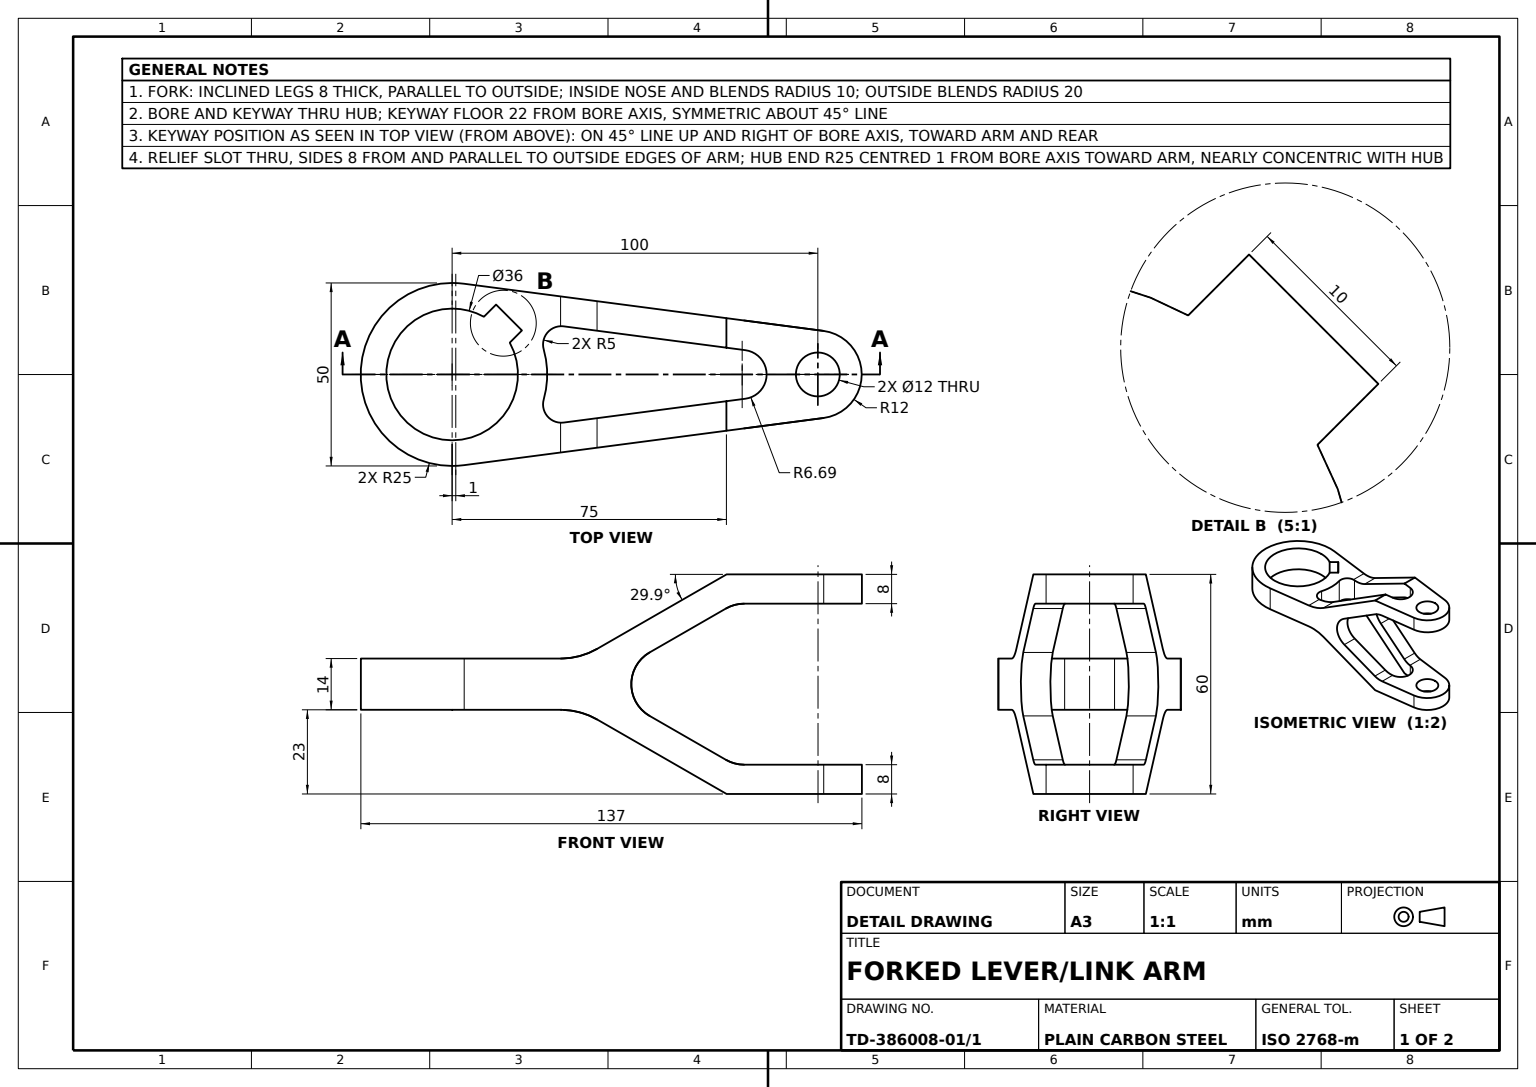
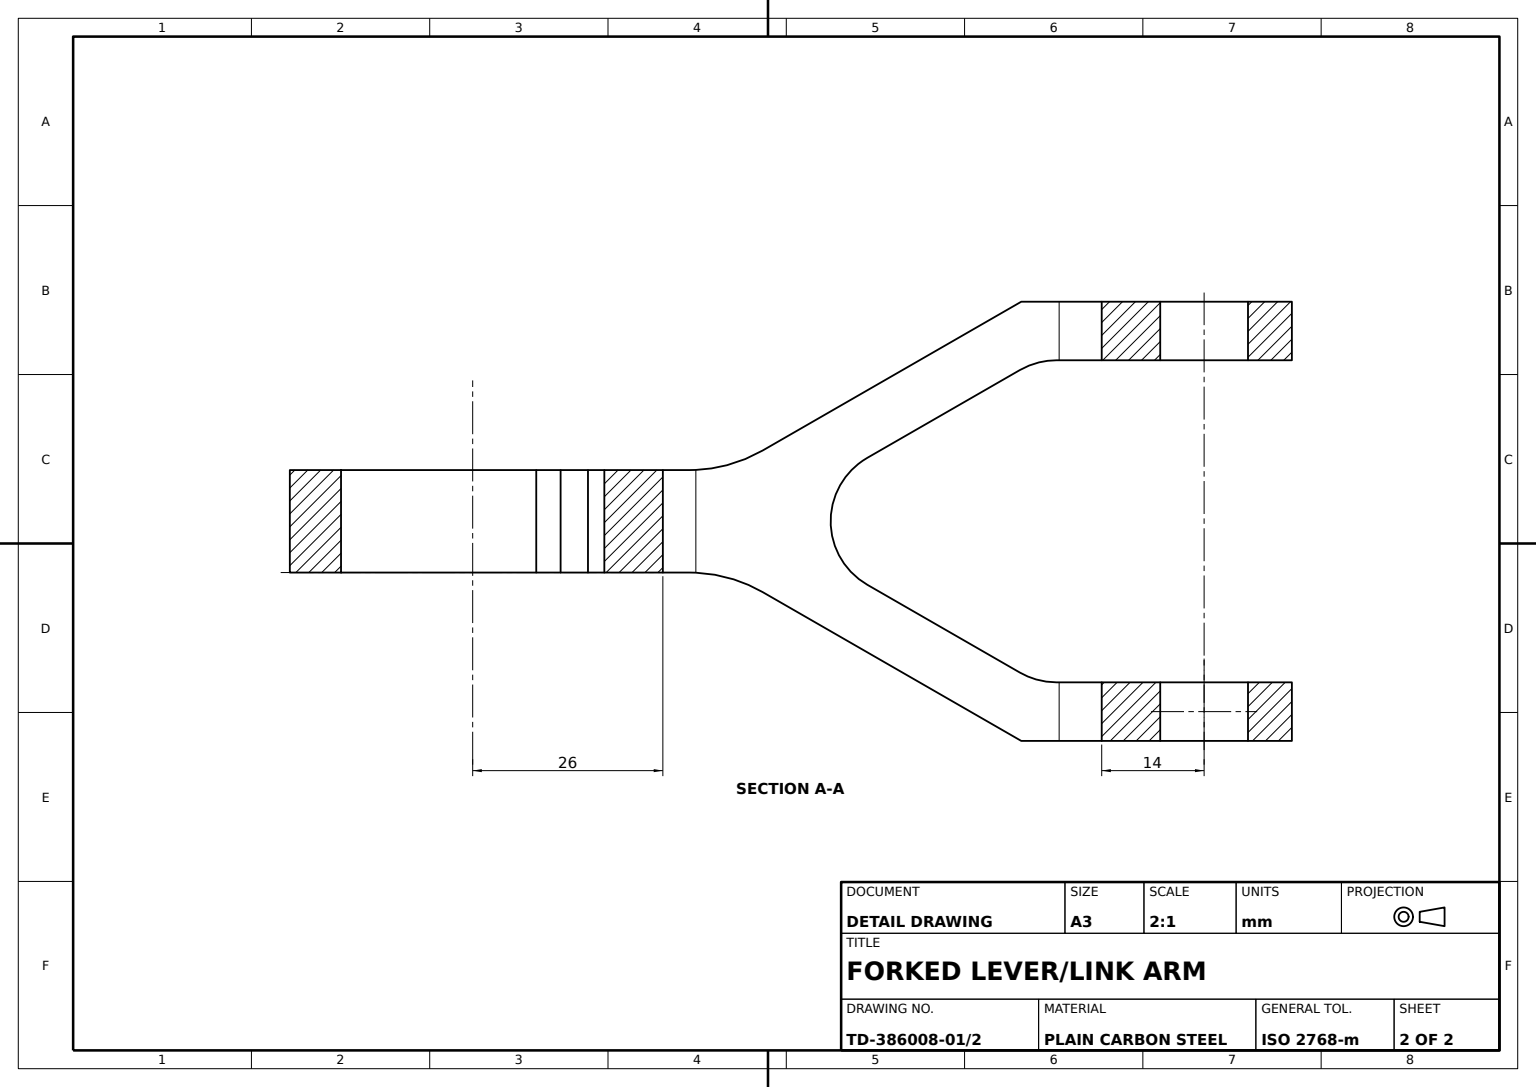
SolidWorks part; units mm, degrees
material "Plain Carbon Steel"
ref_plane "Front Plane" through (0, 0, 0) normal (0, 0, 1) x (1, 0, 0)
ref_plane "Top Plane" through (0, 0, 0) normal (0, 1, 0) x (1, 0, 0)
ref_plane "Right Plane" through (0, 0, 0) normal (1, 0, 0) x (0, 0, -1)
sketch "Side Profile Sketch" plane through (0, 0, 0) normal (0, 1, 0) x (1, 0, 0)
  line L0 (-46.75, 24.7878) -> (51.56, 11.8982)
  line L1 (51.56, -11.8982) -> (-46.75, -24.7878)
  arc A0 (51.56, 11.8982) -> (51.56, -11.8982) centre (50, 0) cw
  arc A1 (-46.75, -24.7878) -> (-46.75, 24.7878) centre (-50, 0) cw
  dimension "D3" = 25
  dimension "D4" = 12
  dimension "D1" = 100
  dimension "D2" = 50
extrude "Lever Blank" add sketch "Side Profile Sketch" against normal mid plane 60
sketch "Hub Bore Sketch" plane through (0, 30, 0) normal (0, 1, 0) x (1, 0, 0)
  line L0 (-1000, 0) -> (49000, 0) construction
  line L1 (-50, -1000) -> (-50, 49000) construction
  line L2 (-50, 0) -> (-15.3108, 34.6892) construction
  line L3 (-41.3085, 15.7626) -> (-37.9792, 19.0919)
  line L4 (-37.9792, 19.0919) -> (-30.9081, 12.0208)
  line L5 (-30.9081, 12.0208) -> (-34.2374, 8.6915)
  arc A0 (-41.3085, 15.7626) -> (-34.2374, 8.6915) centre (-50, 0) ccw
  point P12 (-34.4437, 15.5563)
  dimension "D1" = 36
  dimension "D2" = 22
  dimension "D3" = 10
  dimension "D4" = 5
  dimension "D5" = 45
extrude "Hub Bore Ø36 with Keyway" cut sketch "Hub Bore Sketch" against normal through all
sketch "Hole Ø12 Sketch" plane through (0, 30, 0) normal (0, 1, 0) x (1, 0, 0)
  circle A0 centre (50, 0) radius 6
  dimension "D1" = 12
extrude "Hole Ø12" cut sketch "Hole Ø12 Sketch" against normal through all
sketch "Relief Slot Sketch" plane through (0, 30, 0) normal (0, 1, 0) x (1, 0, 0)
  line L0 (-19.4889, 13.1451) -> (30.18, 6.6329)
  line L1 (30.18, -6.6329) -> (-19.4889, -13.1451)
  line L2 (51.56, 11.8982) -> (-46.75, 24.7878) construction
  line L3 (-46.75, -24.7878) -> (51.56, -11.8982) construction
  arc A0 (30.18, 6.6329) -> (30.18, -6.6329) centre (29.3103, 0) cw
  arc A1 (-19.4889, -13.1451) -> (-24.9491, -6.8229) centre (-20.1389, -8.1875) cw
  arc A2 (-24.9491, -6.8229) -> (-24.9491, 6.8229) centre (-49, 0) ccw
  arc A3 (-24.9491, 6.8229) -> (-19.4889, 13.1451) centre (-20.1389, 8.1875) cw
  arc A4 (-41.3085, 15.7626) -> (-34.2374, 8.6915) centre (-50, 0) ccw construction
  circle A5 centre (50, 0) radius 6 construction
  point P15 (-24, 0)
  point P19 (36, 0)
  dimension "D1" = 5
  dimension "D2" = 5
  dimension "D3" = 26
  dimension "D6" = 25
  dimension "D4" = 8
  dimension "D5" = 14
extrude "Relief Slot" cut sketch "Relief Slot Sketch" against normal through all
sketch "Fork Outline Sketch" plane through (0, 0, 0) normal (0, 0, 1) x (1, 0, 0)
  line L0 (-75, 30) -> (-75, 7)
  line L1 (-75, 30) -> (-75, -30) construction
  line L2 (-75, 7) -> (-20.3401, 7)
  line L3 (-10.3707, 9.6619) -> (25, 30)
  line L4 (-46.75, 30) -> (51.56, 30) construction
  line L5 (25, 30) -> (-75, 30)
  line L6 (-75, -30) -> (-75, -7)
  line L8 (-10.3707, -9.6619) -> (25, -30)
  line L9 (-46.75, -30) -> (51.56, -30) construction
  line L10 (25, -30) -> (-75, -30)
  line L11 (-50, -1000.8017) -> (-50, 48999.1983) construction
  line L12 (-1000, 0) -> (49000, 0) construction
  line L13 (-75, -7) -> (-20.3401, -7)
  arc A0 (-10.3707, 9.6619) -> (-20.3401, 7) centre (-20.3401, 27) cw
  arc A1 (-10.3707, -9.6619) -> (-20.3401, -7) centre (-20.3401, -27) ccw
  point P20 (-50, 23999.1983)
  point P22 (-50, 23999.1983)
  point P25 (-15, 7)
  point P28 (-15, -7)
  dimension "D6" = 20
  dimension "D9" = 20
  dimension "D1" = 23
  dimension "D2" = 23
  dimension "D3" = 50
  dimension "D4" = 35
  dimension "D5" = 35
  dimension "D7" = 75
  dimension "D8" = 75
  dimension "D10" = 23999.1983
extrude "Fork Outline Cut" cut sketch "Fork Outline Sketch" against normal mid plane 60
sketch "Arm Windows Sketch" plane through (0, 0, 0) normal (0, 0, 1) x (1, 0, 0)
  line L0 (62, 22) -> (29.8061, 22)
  line L1 (62, -30) -> (62, 30) construction
  line L2 (24.8214, 20.6691) -> (3.9518, 8.6691)
  line L3 (3.9518, -8.6691) -> (24.8214, -20.6691)
  line L4 (29.8061, -22) -> (62, -22)
  line L5 (62, -22) -> (62, 22)
  line L6 (62, 30) -> (51.56, 30) construction
  line L7 (51.56, -30) -> (62, -30) construction
  line L9 (-10.3707, 9.6619) -> (25, 30) construction
  line L10 (25, -30) -> (-10.3707, -9.6619) construction
  arc A0 (3.9518, 8.6691) -> (3.9518, -8.6691) centre (8.9365, 0) ccw
  arc A1 (29.8061, -22) -> (24.8214, -20.6691) centre (29.8061, -12) cw
  arc A2 (29.8061, 22) -> (24.8214, 20.6691) centre (29.8061, 12) ccw
  dimension "D3" = 10
  dimension "D6" = 10
  dimension "D1" = 8
  dimension "D2" = 8
  dimension "D4" = 8
  dimension "D5" = 8
extrude "Arm Lightening Windows" cut sketch "Arm Windows Sketch" against normal mid plane 60
